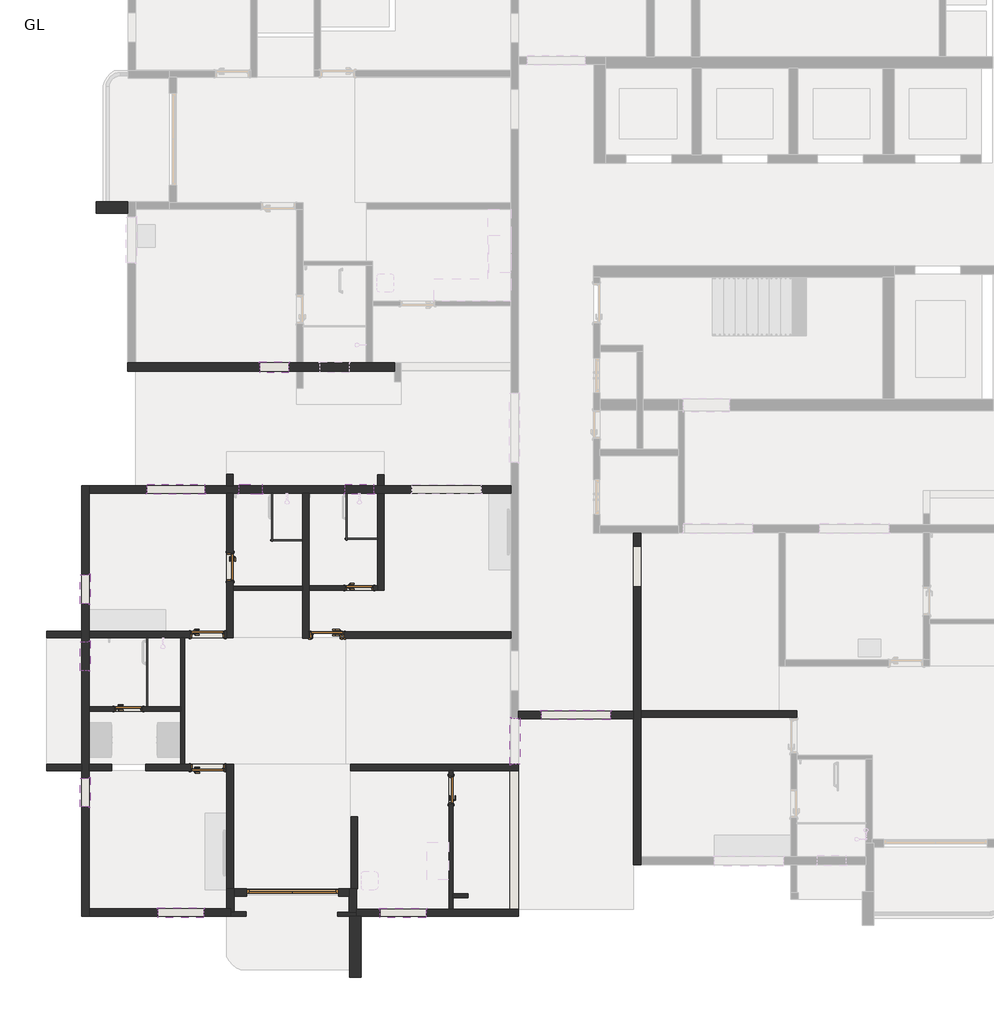
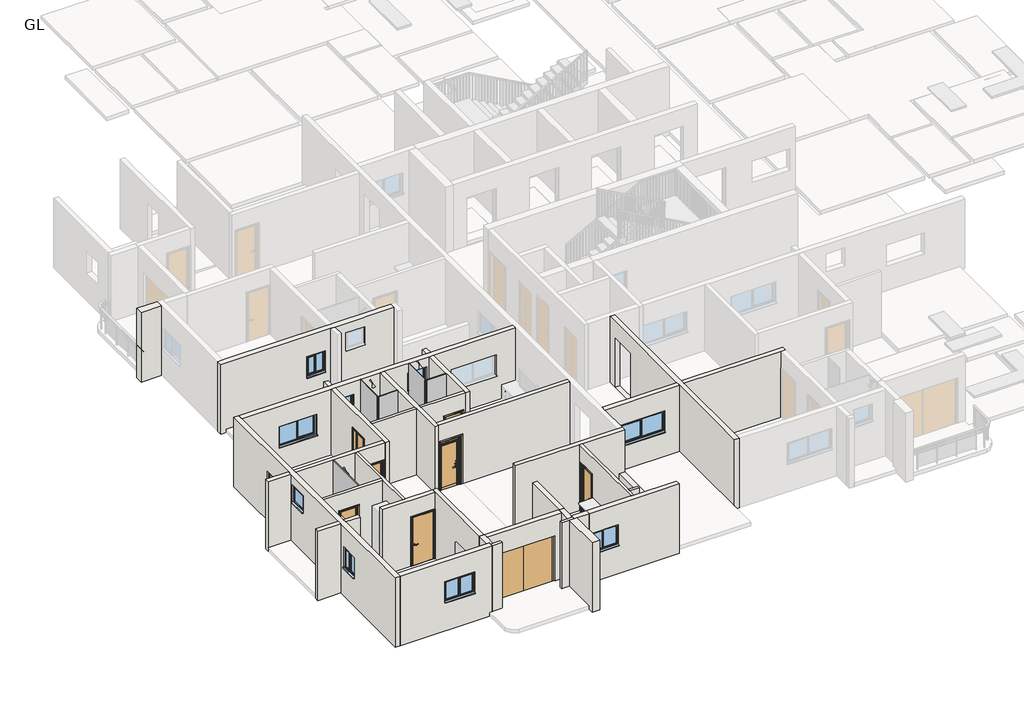
# One storey, part 1 of 14: 36 walls, 11 windows, 9 doors, 5 plates.
"""IFC4 building model written with IfcOpenShell, lengths in millimetres."""

from ifc_helpers import new_model, si_unit, frame, origin, origin_with_axes, place, context, project, spatial, polyline, outline, extrude, faceted_brep, transform, mapped, element, save
from components import doors_concept_extdbl_8_c180431f, doors_intsgl_2_5_door_21b53886, doors_intsgl_2_5_door_ce04bd24, doors_intsgl_2_5_door_1f5f3f16, doors_intsgl_3_door_8261d8fb, doors_intsgl_3_door_f61d7fb9, doors_intsgl_810x2110mm_f0bad3dc, system_panel_glazed_ef83883b, system_panel_glazed_cb88c06f, system_panel_glazed_4b9268f2, system_panel_glazed_6dd91efc, system_panel_glazed_b6b14daa, windows_dbl_plain_2_5_52f1e8c5, windows_dbl_plain_2_5_5b7baf13, windows_dbl_plain_4_4d10fa92, windows_dbl_plain_4_e08ba9e4, windows_dbl_plain_5_c7724a63, windows_dbl_plain_6_decf5736, windows_sgl_plain_2_82341a49, windows_sgl_plain_2_5_9e76a6e6

model = new_model("IFC4")

# Units and contexts
model_context = context("Model", 3, world=origin())
ifc_project = project(units=[si_unit("LENGTHUNIT", "METRE", prefix="MILLI")], contexts=[model_context])

# Site, building, storey
site = spatial("IfcSite", under=ifc_project)
building = spatial("IfcBuilding", under=site)
storey = spatial("IfcBuildingStorey", under=building, Name="GL", Elevation=0.0)

# Doors
placement = place(None, origin())
doors_concept_extdbl_8_shape = doors_concept_extdbl_8_c180431f(model_context)
element("IfcDoor", 1, ObjectType="Doors_Concept_ExtDbl : 8'", at=placement, inside=storey, context=model_context, shape_type="MappedRepresentation", body=[
    mapped(doors_concept_extdbl_8_shape, transform((-11289.2163581, 56773.1334152, 0.0), x_axis=(1.0, 0.0, 0.0), y_axis=(0.0, 1.0, 0.0), z_axis=(0.0, 0.0, 1.0))),
])
doors_intsgl_2_5_door_shape = doors_intsgl_2_5_door_21b53886(model_context)
element("IfcDoor", 2, ObjectType="Doors_IntSgl : 2.5' DOOR", at=placement, inside=storey, context=model_context, shape_type="MappedRepresentation", body=[
    mapped(doors_intsgl_2_5_door_shape, transform((-9514.2506601, 64858.96013, 149.9616), x_axis=(1.0, 0.0, 0.0), y_axis=(0.0, 1.0, 0.0), z_axis=(0.0, 0.0, 1.0))),
])
element("IfcDoor", 3, ObjectType="Doors_IntSgl : 2.5' DOOR", at=placement, inside=storey, context=model_context, shape_type="MappedRepresentation", body=[
    mapped(doors_intsgl_2_5_door_shape, transform((-15646.0698866, 61645.6195727, 149.9616), x_axis=(1.0, 0.0, 0.0), y_axis=(0.0, 1.0, 0.0), z_axis=(0.0, 0.0, 1.0))),
])
doors_intsgl_2_5_door_2_shape = doors_intsgl_2_5_door_ce04bd24(model_context)
element("IfcDoor", 4, ObjectType="Doors_IntSgl : 2.5' DOOR", at=placement, inside=storey, context=model_context, shape_type="MappedRepresentation", body=[
    mapped(doors_intsgl_2_5_door_2_shape, transform((-12951.3420711, 65416.49013, 149.9616), x_axis=(0.0, -1.0, 0.0), y_axis=(1.0, 0.0, 0.0), z_axis=(0.0, 0.0, 1.0))),
])
doors_intsgl_2_5_door_3_shape = doors_intsgl_2_5_door_1f5f3f16(model_context)
element("IfcDoor", 5, ObjectType="Doors_IntSgl : 2.5' DOOR", at=placement, inside=storey, context=model_context, shape_type="MappedRepresentation", body=[
    mapped(doors_intsgl_2_5_door_3_shape, transform((-7083.0672689, 59496.0127724, 149.9616), x_axis=(0.0, 1.0, 0.0), y_axis=(-1.0, 0.0, 0.0), z_axis=(0.0, 0.0, 1.0))),
])
doors_intsgl_3_door_shape = doors_intsgl_3_door_8261d8fb(model_context)
element("IfcDoor", 6, ObjectType="Doors_IntSgl : 3' DOOR", at=placement, inside=storey, context=model_context, shape_type="MappedRepresentation", body=[
    mapped(doors_intsgl_3_door_shape, transform((-13541.6798866, 60093.6754152, 149.9616), x_axis=(1.0, 0.0, 0.0), y_axis=(0.0, 1.0, 0.0), z_axis=(0.0, 0.0, 1.0))),
])
element("IfcDoor", 7, ObjectType="Doors_IntSgl : 3' DOOR", at=placement, inside=storey, context=model_context, shape_type="MappedRepresentation", body=[
    mapped(doors_intsgl_3_door_shape, transform((-10370.9762852, 63608.7807724, 149.9616), x_axis=(-1.0, 0.0, 0.0), y_axis=(0.0, -1.0, 0.0), z_axis=(0.0, 0.0, 1.0))),
])
doors_intsgl_3_door_2_shape = doors_intsgl_3_door_f61d7fb9(model_context)
element("IfcDoor", 8, ObjectType="Doors_IntSgl : 3' DOOR", at=placement, inside=storey, context=model_context, shape_type="MappedRepresentation", body=[
    mapped(doors_intsgl_3_door_2_shape, transform((-13546.2100711, 63618.6686976, 149.9616), x_axis=(1.0, 0.0, 0.0), y_axis=(0.0, 1.0, 0.0), z_axis=(0.0, 0.0, 1.0))),
])
doors_intsgl_810x2110mm_shape = doors_intsgl_810x2110mm_f0bad3dc(model_context)
element("IfcDoor", 9, ObjectType="Doors_IntSgl : 810x2110mm", at=placement, inside=storey, context=model_context, shape_type="MappedRepresentation", body=[
    mapped(doors_intsgl_810x2110mm_shape, transform((-10397.7762852, 63608.7807724, 0.0), x_axis=(-1.0, 0.0, 0.0), y_axis=(0.0, -1.0, 0.0), z_axis=(0.0, 0.0, 1.0))),
])

# Plates
system_panel_glazed_shape = system_panel_glazed_ef83883b(model_context)
element("IfcPlate", 10, ObjectType="System Panel : Glazed", at=placement, inside=storey, context=model_context, shape_type="MappedRepresentation", body=[
    mapped(system_panel_glazed_shape, transform((-11866.147169, 66729.9034152, 0.0), x_axis=(0.0, -1.0, 0.0), y_axis=(1.0, 0.0, 0.0), z_axis=(0.0, 0.0, 1.0))),
])
system_panel_glazed_2_shape = system_panel_glazed_cb88c06f(model_context)
element("IfcPlate", 11, ObjectType="System Panel : Glazed", at=placement, inside=storey, context=model_context, shape_type="MappedRepresentation", body=[
    mapped(system_panel_glazed_2_shape, transform((-11446.7297271, 66092.3334152, 0.0), x_axis=(1.0, 0.0, 0.0), y_axis=(0.0, 1.0, 0.0), z_axis=(0.0, 0.0, 1.0))),
])
system_panel_glazed_3_shape = system_panel_glazed_4b9268f2(model_context)
element("IfcPlate", 12, ObjectType="System Panel : Glazed", at=placement, inside=storey, context=model_context, shape_type="MappedRepresentation", body=[
    mapped(system_panel_glazed_3_shape, transform((-9895.2506601, 66745.1734152, 0.0), x_axis=(0.0, -1.0, 0.0), y_axis=(1.0, 0.0, 0.0), z_axis=(0.0, 0.0, 1.0))),
])
system_panel_glazed_4_shape = system_panel_glazed_6dd91efc(model_context)
element("IfcPlate", 13, ObjectType="System Panel : Glazed", at=placement, inside=storey, context=model_context, shape_type="MappedRepresentation", body=[
    mapped(system_panel_glazed_4_shape, transform((-9463.4506601, 66122.8734152, 0.0), x_axis=(1.0, 0.0, 0.0), y_axis=(0.0, 1.0, 0.0), z_axis=(0.0, 0.0, 1.0))),
])
system_panel_glazed_5_shape = system_panel_glazed_b6b14daa(model_context)
element("IfcPlate", 14, ObjectType="System Panel : Glazed", at=placement, inside=storey, context=model_context, shape_type="MappedRepresentation", body=[
    mapped(system_panel_glazed_5_shape, transform((-15187.4698866, 62623.3346976, 0.0), x_axis=(0.0, -1.0, 0.0), y_axis=(1.0, 0.0, 0.0), z_axis=(0.0, 0.0, 1.0))),
])

# Walls
element("IfcWall", 15, ObjectType="W2", at=placement, inside=storey, context=model_context, shape_type="Brep", body=[
    faceted_brep([(-5294.6931346, 60177.7487724, 3000.0), (-5294.6931346, 60177.7487724, 2110.0), (-5294.6931346, 60177.7487724, 1200.0), (-5294.6931346, 60177.7487724, 0.0), (-5492.8131346, 60177.7487724, 0.0), (-9752.3931346, 60177.7487724, 0.0), (-9752.3931346, 60177.7487724, 3000.0), (-5492.8131346, 60177.7487724, 3000.0), (-5294.6931346, 60004.0127724, 0.0), (-5294.6931346, 60004.0127724, 3000.0), (-7025.9172689, 60004.0127724, 3000.0), (-7140.2172689, 60004.0127724, 3000.0), (-9752.3931346, 60004.0127724, 3000.0), (-9752.3931346, 60004.0127724, 0.0), (-7140.2172689, 60004.0127724, 0.0), (-7025.9172689, 60004.0127724, 0.0), (-5520.9672689, 60004.0127724, 0.0)], [[[0, 1, 2, 3, 4, 5, 6, 7]], [[8, 9, 10, 11, 12, 13, 14, 15, 16]], [[5, 4, 3, 8, 16, 15, 14, 13]], [[6, 5, 13, 12]], [[0, 7, 6, 12, 11, 10, 9]], [[0, 9, 8, 3, 2, 1]]]),
])
element("IfcWall", 16, ObjectType="W2", at=placement, inside=storey, context=model_context, shape_type="Brep", body=[
    faceted_brep([(-9742.8728296, 58794.5197223, 0.0), (-9742.8728296, 56872.1934152, 0.0), (-9742.8728296, 56872.1934152, 3000.0), (-9742.8728296, 58794.5197223, 3000.0), (-9569.1368296, 58794.5197223, 0.0), (-9569.1368296, 58794.5197223, 3000.0), (-9569.1368296, 56872.1934152, 3000.0), (-9569.1368296, 56872.1934152, 0.0), (-9585.6556011, 56872.1934152, 0.0), (-9585.6556011, 56872.1934152, 3000.0)], [[[0, 1, 2, 3]], [[4, 5, 6, 7]], [[1, 0, 4, 7, 8]], [[3, 2, 9, 6, 5]], [[0, 3, 5, 4]], [[2, 1, 8, 7, 6, 9]]]),
])
element("IfcWall", 17, ObjectType="W2", at=placement, inside=storey, context=model_context, shape_type="Brep", body=[
    faceted_brep([(-12859.9438866, 56872.1934152, 0.0), (-12859.9438866, 60180.5434152, 0.0), (-12859.9438866, 60180.5434152, 3000.0), (-12859.9438866, 56872.1934152, 3000.0), (-13033.6798866, 56872.1934152, 0.0), (-13033.6798866, 56872.1934152, 3000.0), (-13033.6798866, 60006.8074152, 3000.0), (-13033.6798866, 60180.5434152, 3000.0), (-13033.6798866, 60180.5434152, 0.0), (-13033.6798866, 60006.8074152, 0.0)], [[[0, 1, 2, 3]], [[4, 5, 6, 7, 8, 9]], [[1, 0, 4, 9, 8]], [[3, 2, 7, 6, 5]], [[0, 3, 5, 4]], [[2, 1, 8, 7]]]),
])
element("IfcWall", 18, ObjectType="W2", at=placement, inside=storey, context=model_context, shape_type="Brep", body=[
    faceted_brep([(-13033.6798866, 60180.5434152, 0.0), (-14151.3407376, 60180.5434152, 0.0), (-14265.6407376, 60180.5434152, 0.0), (-15194.7118866, 60180.5434152, 0.0), (-15194.7118866, 60180.5434152, 3000.0), (-14265.6407376, 60180.5434152, 3000.0), (-14151.3407376, 60180.5434152, 3000.0), (-13033.6798866, 60180.5434152, 3000.0), (-13084.4798866, 60180.5434152, 149.9616), (-13084.4798866, 60180.5434152, 2259.9616), (-13998.8798866, 60180.5434152, 2259.9616), (-13998.8798866, 60180.5434152, 149.9616), (-15194.7118866, 60006.8074152, 0.0), (-13033.6798866, 60006.8074152, 0.0), (-13033.6798866, 60006.8074152, 3000.0), (-15194.7118866, 60006.8074152, 3000.0), (-13084.4798866, 60006.8074152, 2259.9616), (-13084.4798866, 60006.8074152, 149.9616), (-13998.8798866, 60006.8074152, 149.9616), (-13998.8798866, 60006.8074152, 2259.9616)], [[[0, 1, 2, 3, 4, 5, 6, 7], [8, 9, 10, 11]], [[12, 13, 14, 15], [16, 17, 18, 19]], [[3, 2, 1, 0, 13, 12]], [[4, 3, 12, 15]], [[7, 6, 5, 4, 15, 14]], [[0, 7, 14, 13]], [[8, 17, 16, 9]], [[9, 16, 19, 10]], [[10, 19, 18, 11]], [[17, 8, 11, 18]]]),
])
element("IfcWall", 19, ObjectType="W2", at=placement, inside=storey, context=model_context, shape_type="SweptSolid", body=[
    extrude(outline(polyline([(-17819.0398866, 63705.5366976), (-16889.3998866, 63705.5366976), (-16889.3998866, 63531.8006976), (-17819.0398866, 63531.8006976), (-17819.0398866, 63705.5366976)])), origin_with_axes(), (0.0, 0.0, 1.0), 3000.0),
])
element("IfcWall", 20, ObjectType="W2", at=placement, inside=storey, context=model_context, shape_type="Brep", body=[
    faceted_brep([(-13038.2100711, 67367.4734152, 0.0), (-13038.2100711, 63705.5366976, 0.0), (-13038.2100711, 63531.8006976, 0.0), (-13038.2100711, 63531.8006976, 3000.0), (-13038.2100711, 63705.5366976, 3000.0), (-13038.2100711, 67367.4734152, 3000.0), (-13038.2100711, 65035.49013, 2259.9616), (-13038.2100711, 65035.49013, 149.9616), (-13038.2100711, 65797.49013, 149.9616), (-13038.2100711, 65797.49013, 2259.9616), (-12864.4740711, 63531.8006976, 0.0), (-12864.4740711, 64794.19013, 0.0), (-12864.4740711, 64908.49013, 0.0), (-12864.4740711, 67367.4734152, 0.0), (-12864.4740711, 67367.4734152, 3000.0), (-12864.4740711, 64908.49013, 3000.0), (-12864.4740711, 64794.19013, 3000.0), (-12864.4740711, 63531.8006976, 3000.0), (-12864.4740711, 65035.49013, 149.9616), (-12864.4740711, 65035.49013, 2259.9616), (-12864.4740711, 65797.49013, 2259.9616), (-12864.4740711, 65797.49013, 149.9616)], [[[0, 1, 2, 3, 4, 5], [6, 7, 8, 9]], [[10, 11, 12, 13, 14, 15, 16, 17], [18, 19, 20, 21]], [[2, 1, 0, 13, 12, 11, 10]], [[5, 4, 3, 17, 16, 15, 14]], [[0, 5, 14, 13]], [[3, 2, 10, 17]], [[18, 7, 6, 19]], [[19, 6, 9, 20]], [[20, 9, 8, 21]], [[7, 18, 21, 8]]]),
])
element("IfcWall", 21, ObjectType="W2", at=placement, inside=storey, context=model_context, shape_type="Brep", body=[
    faceted_brep([(-11027.3122852, 67367.4734152, 0.0), (-11027.3122852, 64908.49013, 0.0), (-11027.3122852, 64794.19013, 0.0), (-11027.3122852, 63521.9127724, 0.0), (-11027.3122852, 63521.9127724, 3000.0), (-11027.3122852, 64794.19013, 3000.0), (-11027.3122852, 64908.49013, 3000.0), (-11027.3122852, 67367.4734152, 3000.0), (-10853.5762852, 67367.4734152, 0.0), (-10853.5762852, 67367.4734152, 3000.0), (-10853.5762852, 64916.11013, 3000.0), (-10853.5762852, 64801.81013, 3000.0), (-10853.5762852, 63695.6487724, 3000.0), (-10853.5762852, 63521.9127724, 3000.0), (-10853.5762852, 63521.9127724, 0.0), (-10853.5762852, 63695.6487724, 0.0), (-10853.5762852, 64801.81013, 0.0), (-10853.5762852, 64916.11013, 0.0)], [[[0, 1, 2, 3, 4, 5, 6, 7]], [[8, 9, 10, 11, 12, 13, 14, 15, 16, 17]], [[3, 2, 1, 0, 8, 17, 16, 15, 14]], [[7, 6, 5, 4, 13, 12, 11, 10, 9]], [[0, 7, 9, 8]], [[4, 3, 14, 13]]]),
])
element("IfcWall", 22, ObjectType="W2", at=placement, inside=storey, context=model_context, shape_type="Brep", body=[
    faceted_brep([(-9031.6506601, 67367.4734152, 0.0), (-9031.6506601, 64916.11013, 0.0), (-9031.6506601, 64801.81013, 0.0), (-9031.6506601, 64801.81013, 3000.0), (-9031.6506601, 64916.11013, 3000.0), (-9031.6506601, 67367.4734152, 3000.0), (-8857.9146601, 67367.4734152, 0.0), (-8857.9146601, 67367.4734152, 3000.0), (-8857.9146601, 64801.81013, 3000.0), (-8857.9146601, 64801.81013, 0.0)], [[[0, 1, 2, 3, 4, 5]], [[6, 7, 8, 9]], [[2, 1, 0, 6, 9]], [[5, 4, 3, 8, 7]], [[0, 5, 7, 6]], [[3, 2, 9, 8]]]),
])
element("IfcWall", 23, ObjectType="W2", at=placement, inside=storey, context=model_context, shape_type="SweptSolid", body=[
    extrude(outline(polyline([(3000.0, -5492.8131346), (3000.0, -10853.5762852), (0.0, -10853.5762852), (0.0, -10802.7762852), (149.9616, -10802.7762852), (149.9616, -10828.1762852), (2259.9616, -10828.1762852), (2259.9616, -9913.7762852), (149.9616, -9913.7762852), (149.9616, -9992.7762852), (0.0, -9992.7762852), (0.0, -5492.8131346), (3000.0, -5492.8131346)])), frame((0.0, 63521.9127724, 0.0), z_axis=(0.0, 1.0, 0.0), x_axis=(0.0, 0.0, 1.0)), (0.0, 0.0, 1.0), 173.736),
])
element("IfcWall", 24, ObjectType="W2", at=placement, inside=storey, context=model_context, shape_type="Brep", body=[
    faceted_brep([(-16691.2798866, 63531.8006976, 0.0), (-14265.6407376, 63531.8006976, 0.0), (-14151.3407376, 63531.8006976, 0.0), (-13038.2100711, 63531.8006976, 0.0), (-13038.2100711, 63531.8006976, 3000.0), (-14151.3407376, 63531.8006976, 3000.0), (-14265.6407376, 63531.8006976, 3000.0), (-16691.2798866, 63531.8006976, 3000.0), (-13089.0100711, 63531.8006976, 2259.9616), (-13089.0100711, 63531.8006976, 149.9616), (-14003.4100711, 63531.8006976, 149.9616), (-14003.4100711, 63531.8006976, 2259.9616), (-13038.2100711, 63705.5366976, 0.0), (-16691.2798866, 63705.5366976, 0.0), (-16691.2798866, 63705.5366976, 3000.0), (-13038.2100711, 63705.5366976, 3000.0), (-13089.0100711, 63705.5366976, 149.9616), (-13089.0100711, 63705.5366976, 2259.9616), (-14003.4100711, 63705.5366976, 2259.9616), (-14003.4100711, 63705.5366976, 149.9616)], [[[0, 1, 2, 3, 4, 5, 6, 7], [8, 9, 10, 11]], [[12, 13, 14, 15], [16, 17, 18, 19]], [[3, 2, 1, 0, 13, 12]], [[7, 6, 5, 4, 15, 14]], [[0, 7, 14, 13]], [[4, 3, 12, 15]], [[16, 9, 8, 17]], [[17, 8, 11, 18]], [[18, 11, 10, 19]], [[9, 16, 19, 10]]]),
])
element("IfcWall", 25, ObjectType="W2", at=placement, inside=storey, context=model_context, shape_type="SweptSolid", body=[
    extrude(outline(polyline([(-17820.0558866, 60006.8074152), (-17820.0558866, 60180.5434152), (-16889.3998866, 60180.5434152), (-16889.3998866, 60006.8074152), (-17820.0558866, 60006.8074152)])), origin_with_axes(), (0.0, 0.0, 1.0), 3000.0),
    extrude(outline(polyline([(-16092.8558866, 60180.5434152), (-16092.8558866, 60006.8074152), (-16691.2798866, 60006.8074152), (-16691.2798866, 60180.5434152), (-16092.8558866, 60180.5434152)])), origin_with_axes(), (0.0, 0.0, 1.0), 3000.0),
])
element("IfcWall", 26, ObjectType="W2", at=placement, inside=storey, context=model_context, shape_type="SweptSolid", body=[
    extrude(outline(polyline([(-12864.4740711, 67870.3934152), (-12864.4740711, 67565.5934152), (-13038.2100711, 67565.5934152), (-13038.2100711, 67870.3934152), (-12864.4740711, 67870.3934152)])), origin_with_axes(), (0.0, 0.0, 1.0), 3000.0),
])
element("IfcWall", 27, ObjectType="W2", at=placement, inside=storey, context=model_context, shape_type="SweptSolid", body=[
    extrude(outline(polyline([(-8857.9146601, 67864.0434152), (-8857.9146601, 67565.5934152), (-9031.6506601, 67565.5934152), (-9031.6506601, 67864.0434152), (-8857.9146601, 67864.0434152)])), origin_with_axes(), (0.0, 0.0, 1.0), 3000.0),
])
element("IfcWall", 28, ObjectType="W2", at=placement, inside=storey, context=model_context, shape_type="Brep", body=[
    faceted_brep([(-2044.3665436, 61430.4767724, 0.0), (1930.5893567, 61430.4767724, 0.0), (2098.2293567, 61430.4767724, 0.0), (2098.2293567, 61430.4767724, 3000.0), (1930.5893567, 61430.4767724, 3000.0), (-2044.3665436, 61430.4767724, 3000.0), (-2044.3665436, 61604.2127724, 0.0), (-2044.3665436, 61604.2127724, 3000.0), (2098.2293567, 61604.2127724, 3000.0), (2098.2293567, 61604.2127724, 0.0)], [[[0, 1, 2, 3, 4, 5]], [[6, 7, 8, 9]], [[2, 1, 0, 6, 9]], [[5, 4, 3, 8, 7]], [[0, 5, 7, 6]], [[3, 2, 9, 8]]]),
])
element("IfcWall", 29, ObjectType="W3", at=placement, inside=storey, context=model_context, shape_type="SweptSolid", body=[
    extrude(outline(polyline([(0.0, -10853.5762852), (0.0, -9031.6506601), (3000.0, -9031.6506601), (3000.0, -10853.5762852), (0.0, -10853.5762852)]), holes=[polyline([(2259.9616, -9133.2506601), (149.9616, -9133.2506601), (149.9616, -9895.2506601), (2259.9616, -9895.2506601), (2259.9616, -9133.2506601)])]), frame((0.0, 64801.81013, 0.0), z_axis=(0.0, 1.0, 0.0), x_axis=(0.0, 0.0, 1.0)), (0.0, 0.0, 1.0), 114.3),
])
element("IfcWall", 30, ObjectType="W3", at=placement, inside=storey, context=model_context, shape_type="SweptSolid", body=[
    extrude(outline(polyline([(-12864.4740711, 64908.49013), (-11027.3122852, 64908.49013), (-11027.3122852, 64794.19013), (-12864.4740711, 64794.19013), (-12864.4740711, 64908.49013)])), origin_with_axes(), (0.0, 0.0, 1.0), 3000.0),
])
element("IfcWall", 31, ObjectType="W3", at=placement, inside=storey, context=model_context, shape_type="Brep", body=[
    faceted_brep([(-14265.6407376, 63531.8006976, 0.0), (-14265.6407376, 61702.7695727, 0.0), (-14265.6407376, 61588.4695727, 0.0), (-14265.6407376, 60180.5434152, 0.0), (-14265.6407376, 60180.5434152, 3000.0), (-14265.6407376, 61588.4695727, 3000.0), (-14265.6407376, 61702.7695727, 3000.0), (-14265.6407376, 63531.8006976, 3000.0), (-14151.3407376, 63531.8006976, 0.0), (-14151.3407376, 63531.8006976, 3000.0), (-14151.3407376, 60180.5434152, 3000.0), (-14151.3407376, 60180.5434152, 0.0)], [[[0, 1, 2, 3, 4, 5, 6, 7]], [[8, 9, 10, 11]], [[3, 2, 1, 0, 8, 11]], [[7, 6, 5, 4, 10, 9]], [[4, 3, 11, 10]], [[0, 7, 9, 8]]]),
])
element("IfcWall", 32, ObjectType="W3", at=placement, inside=storey, context=model_context, shape_type="SweptSolid", body=[
    extrude(outline(polyline([(0.0, -16691.2798866), (0.0, -14265.6407376), (3000.0, -14265.6407376), (3000.0, -16691.2798866), (0.0, -16691.2798866)]), holes=[polyline([(2259.9616, -15265.0698866), (149.9616, -15265.0698866), (149.9616, -16027.0698866), (2259.9616, -16027.0698866), (2259.9616, -15265.0698866)])]), frame((0.0, 61588.4695727, 0.0), z_axis=(0.0, 1.0, 0.0), x_axis=(0.0, 0.0, 1.0)), (0.0, 0.0, 1.0), 114.3),
])
element("IfcWall", 33, ObjectType="W3", at=placement, inside=storey, context=model_context, shape_type="Brep", body=[
    faceted_brep([(-12524.4098866, 56265.3874152, 0.0), (-12835.5598866, 56265.3874152, 0.0), (-12934.6198866, 56265.3874152, 0.0), (-12934.6198866, 56265.3874152, 3000.0), (-12835.5598866, 56265.3874152, 3000.0), (-12524.4098866, 56265.3874152, 3000.0), (-12524.4098866, 56151.0874152, 0.0), (-12524.4098866, 56151.0874152, 3000.0), (-12934.6198866, 56151.0874152, 3000.0), (-12934.6198866, 56151.0874152, 0.0)], [[[0, 1, 2, 3, 4, 5]], [[6, 7, 8, 9]], [[2, 1, 0, 6, 9]], [[3, 2, 9, 8]], [[5, 4, 3, 8, 7]], [[0, 5, 7, 6]]]),
])
element("IfcWall", 34, ObjectType="W3", at=placement, inside=storey, context=model_context, shape_type="Brep", body=[
    faceted_brep([(-9585.6556011, 56257.2296151, 0.0), (-9783.7756011, 56257.2296151, 0.0), (-10094.9256011, 56257.2296151, 0.0), (-10094.9256011, 56257.2296151, 3000.0), (-9783.7756011, 56257.2296151, 3000.0), (-9585.6556011, 56257.2296151, 3000.0), (-9585.6556011, 56142.9296151, 0.0), (-9585.6556011, 56142.9296151, 3000.0), (-9782.0683526, 56142.9296151, 3000.0), (-10094.9256011, 56142.9296151, 3000.0), (-10094.9256011, 56142.9296151, 0.0), (-9782.0683526, 56142.9296151, 0.0)], [[[0, 1, 2, 3, 4, 5]], [[6, 7, 8, 9, 10, 11]], [[2, 1, 0, 6, 11, 10]], [[3, 2, 10, 9]], [[5, 4, 3, 9, 8, 7]], [[0, 5, 7, 6]]]),
])
element("IfcWall", 35, ObjectType="W3", at=placement, inside=storey, context=model_context, shape_type="Brep", body=[
    faceted_brep([(-7025.9172689, 56341.0496151, 0.0), (-7025.9172689, 56636.5035386, 0.0), (-7025.9172689, 56750.8035386, 0.0), (-7025.9172689, 60004.0127724, 0.0), (-7025.9172689, 60004.0127724, 3000.0), (-7025.9172689, 56750.8035386, 3000.0), (-7025.9172689, 56636.5035386, 3000.0), (-7025.9172689, 56341.0496151, 3000.0), (-7025.9172689, 59877.0127724, 2259.9616), (-7025.9172689, 59877.0127724, 149.9616), (-7025.9172689, 59115.0127724, 149.9616), (-7025.9172689, 59115.0127724, 2259.9616), (-7140.2172689, 60004.0127724, 0.0), (-7140.2172689, 56341.0496151, 0.0), (-7140.2172689, 56341.0496151, 3000.0), (-7140.2172689, 60004.0127724, 3000.0), (-7140.2172689, 59877.0127724, 149.9616), (-7140.2172689, 59877.0127724, 2259.9616), (-7140.2172689, 59115.0127724, 2259.9616), (-7140.2172689, 59115.0127724, 149.9616)], [[[0, 1, 2, 3, 4, 5, 6, 7], [8, 9, 10, 11]], [[12, 13, 14, 15], [16, 17, 18, 19]], [[3, 2, 1, 0, 13, 12]], [[7, 6, 5, 4, 15, 14]], [[4, 3, 12, 15]], [[0, 7, 14, 13]], [[16, 9, 8, 17]], [[17, 8, 11, 18]], [[18, 11, 10, 19]], [[9, 16, 19, 10]]]),
])
element("IfcWall", 36, ObjectType="W3", at=placement, inside=storey, context=model_context, shape_type="SweptSolid", body=[
    extrude(outline(polyline([(-6632.2172689, 56636.5035386), (-7025.9172689, 56636.5035386), (-7025.9172689, 56750.8035386), (-6632.2172689, 56750.8035386), (-6632.2172689, 56636.5035386)])), origin_with_axes(), (0.0, 0.0, 1.0), 3000.0),
])
element("IfcWall", 37, ObjectType="W4", at=placement, inside=storey, context=model_context, shape_type="Brep", body=[
    faceted_brep([(-9477.2683526, 54525.5707921, 0.0), (-9477.2683526, 56142.9296151, 0.0), (-9477.2683526, 56142.9296151, 3000.0), (-9477.2683526, 54525.5707921, 3000.0), (-9782.0683526, 54525.5707921, 0.0), (-9782.0683526, 54525.5707921, 3000.0), (-9782.0683526, 56142.9296151, 3000.0), (-9782.0683526, 56142.9296151, 0.0), (-9585.6556011, 56142.9296151, 0.0), (-9585.6556011, 56142.9296151, 3000.0)], [[[0, 1, 2, 3]], [[4, 5, 6, 7]], [[1, 0, 4, 7, 8]], [[3, 2, 9, 6, 5]], [[0, 3, 5, 4]], [[2, 1, 8, 7, 6, 9]]]),
])
element("IfcWall", 38, ObjectType="W4", at=placement, inside=storey, context=model_context, shape_type="SweptSolid", body=[
    extrude(outline(polyline([(-15665.5131346, 74800.7827724), (-16503.7131346, 74800.7827724), (-16503.7131346, 75105.5827724), (-15665.5131346, 75105.5827724), (-15665.5131346, 74800.7827724)])), origin_with_axes(), (0.0, 0.0, 1.0), 3000.0),
])
element("IfcWall", 39, ObjectType="W5", at=placement, inside=storey, context=model_context, shape_type="Brep", body=[
    faceted_brep([(-5292.3672689, 56341.0496151, 0.0), (-5292.3672689, 60004.0127724, 0.0), (-5292.3672689, 60004.0127724, 1171.2), (-5292.3672689, 56341.0496151, 1171.2), (-5520.9672689, 56341.0496151, 0.0), (-5520.9672689, 56341.0496151, 1171.2), (-5520.9672689, 60004.0127724, 1171.2), (-5520.9672689, 60004.0127724, 0.0), (-5294.6931346, 60004.0127724, 0.0)], [[[0, 1, 2, 3]], [[4, 5, 6, 7]], [[1, 0, 4, 7, 8]], [[3, 2, 6, 5]], [[0, 3, 5, 4]], [[2, 1, 8, 7, 6]]]),
])
element("IfcWall", 40, ObjectType="W5", at=placement, inside=storey, context=model_context, shape_type="Brep", body=[
    faceted_brep([(-8587.5491346, 70838.3827724, 0.0), (-9163.1131346, 70838.3827724, 0.0), (-9336.8491346, 70838.3827724, 0.0), (-11010.9631346, 70838.3827724, 0.0), (-11178.6031346, 70838.3827724, 0.0), (-15452.1531346, 70838.3827724, 0.0), (-15665.5131346, 70838.3827724, 0.0), (-15665.5131346, 70838.3827724, 3000.0), (-15452.1531346, 70838.3827724, 3000.0), (-11178.6031346, 70838.3827724, 3000.0), (-11010.9631346, 70838.3827724, 3000.0), (-9336.8491346, 70838.3827724, 3000.0), (-9163.1131346, 70838.3827724, 3000.0), (-8587.5491346, 70838.3827724, 3000.0), (-9794.0491346, 70838.3827724, 2590.8), (-10556.0491346, 70838.3827724, 2590.8), (-10556.0491346, 70838.3827724, 1828.8), (-9794.0491346, 70838.3827724, 1828.8), (-11394.2491346, 70838.3827724, 2110.0), (-12156.2491346, 70838.3827724, 2110.0), (-12156.2491346, 70838.3827724, 1200.0), (-11394.2491346, 70838.3827724, 1200.0), (-8587.5491346, 70609.7827724, 0.0), (-8587.5491346, 70609.7827724, 3000.0), (-11010.9631346, 70609.7827724, 3000.0), (-11178.6031346, 70609.7827724, 3000.0), (-15665.5131346, 70609.7827724, 3000.0), (-15665.5131346, 70609.7827724, 0.0), (-11178.6031346, 70609.7827724, 0.0), (-11010.9631346, 70609.7827724, 0.0), (-9794.0491346, 70609.7827724, 2590.8), (-9794.0491346, 70609.7827724, 1828.8), (-10556.0491346, 70609.7827724, 1828.8), (-10556.0491346, 70609.7827724, 2590.8), (-11394.2491346, 70609.7827724, 2110.0), (-11394.2491346, 70609.7827724, 1200.0), (-12156.2491346, 70609.7827724, 1200.0), (-12156.2491346, 70609.7827724, 2110.0)], [[[0, 1, 2, 3, 4, 5, 6, 7, 8, 9, 10, 11, 12, 13], [14, 15, 16, 17], [18, 19, 20, 21]], [[22, 23, 24, 25, 26, 27, 28, 29], [30, 31, 32, 33], [34, 35, 36, 37]], [[6, 5, 4, 3, 2, 1, 0, 22, 29, 28, 27]], [[13, 12, 11, 10, 9, 8, 7, 26, 25, 24, 23]], [[7, 6, 27, 26]], [[31, 30, 14, 17]], [[32, 31, 17, 16]], [[33, 32, 16, 15]], [[30, 33, 15, 14]], [[35, 34, 18, 21]], [[36, 35, 21, 20]], [[37, 36, 20, 19]], [[34, 37, 19, 18]], [[0, 13, 23, 22]]]),
])
element("IfcWall", 41, ObjectType="WALL 1", at=placement, inside=storey, context=model_context, shape_type="Brep", body=[
    faceted_brep([(-16691.2798866, 56151.0874152, 0.0), (-16691.2798866, 56349.2074152, 0.0), (-16691.2798866, 60006.8074152, 0.0), (-16691.2798866, 60180.5434152, 0.0), (-16691.2798866, 61588.4695727, 0.0), (-16691.2798866, 61702.7695727, 0.0), (-16691.2798866, 63531.8006976, 0.0), (-16691.2798866, 63705.5366976, 0.0), (-16691.2798866, 67367.4734152, 0.0), (-16691.2798866, 67565.5934152, 0.0), (-16691.2798866, 67565.5934152, 3000.0), (-16691.2798866, 67367.4734152, 3000.0), (-16691.2798866, 63705.5366976, 3000.0), (-16691.2798866, 63531.8006976, 3000.0), (-16691.2798866, 61702.7695727, 3000.0), (-16691.2798866, 61588.4695727, 3000.0), (-16691.2798866, 60180.5434152, 3000.0), (-16691.2798866, 60006.8074152, 3000.0), (-16691.2798866, 56349.2074152, 3000.0), (-16691.2798866, 56151.0874152, 3000.0), (-16691.2798866, 59048.4695727, 2110.0), (-16691.2798866, 59810.4695727, 2110.0), (-16691.2798866, 59810.4695727, 1200.0), (-16691.2798866, 59048.4695727, 1200.0), (-16691.2798866, 62668.2006976, 2590.8), (-16691.2798866, 63430.2006976, 2590.8), (-16691.2798866, 63430.2006976, 1828.8), (-16691.2798866, 62668.2006976, 1828.8), (-16691.2798866, 64442.1366976, 2110.0), (-16691.2798866, 65204.1366976, 2110.0), (-16691.2798866, 65204.1366976, 1200.0), (-16691.2798866, 64442.1366976, 1200.0), (-16889.3998866, 56151.0874152, 0.0), (-16889.3998866, 56151.0874152, 3000.0), (-16889.3998866, 60006.8074152, 3000.0), (-16889.3998866, 60180.5434152, 3000.0), (-16889.3998866, 63531.8006976, 3000.0), (-16889.3998866, 63705.5366976, 3000.0), (-16889.3998866, 67565.5934152, 3000.0), (-16889.3998866, 67565.5934152, 0.0), (-16889.3998866, 63705.5366976, 0.0), (-16889.3998866, 63531.8006976, 0.0), (-16889.3998866, 60180.5434152, 0.0), (-16889.3998866, 60006.8074152, 0.0), (-16889.3998866, 59048.4695727, 2110.0), (-16889.3998866, 59048.4695727, 1200.0), (-16889.3998866, 59810.4695727, 1200.0), (-16889.3998866, 59810.4695727, 2110.0), (-16889.3998866, 62668.2006976, 2590.8), (-16889.3998866, 62668.2006976, 1828.8), (-16889.3998866, 63430.2006976, 1828.8), (-16889.3998866, 63430.2006976, 2590.8), (-16889.3998866, 64442.1366976, 2110.0), (-16889.3998866, 64442.1366976, 1200.0), (-16889.3998866, 65204.1366976, 1200.0), (-16889.3998866, 65204.1366976, 2110.0)], [[[0, 1, 2, 3, 4, 5, 6, 7, 8, 9, 10, 11, 12, 13, 14, 15, 16, 17, 18, 19], [20, 21, 22, 23], [24, 25, 26, 27], [28, 29, 30, 31]], [[32, 33, 34, 35, 36, 37, 38, 39, 40, 41, 42, 43], [44, 45, 46, 47], [48, 49, 50, 51], [52, 53, 54, 55]], [[9, 8, 7, 6, 5, 4, 3, 2, 1, 0, 32, 43, 42, 41, 40, 39]], [[19, 18, 17, 16, 15, 14, 13, 12, 11, 10, 38, 37, 36, 35, 34, 33]], [[0, 19, 33, 32]], [[10, 9, 39, 38]], [[45, 44, 20, 23]], [[46, 45, 23, 22]], [[47, 46, 22, 21]], [[44, 47, 21, 20]], [[49, 48, 24, 27]], [[50, 49, 27, 26]], [[51, 50, 26, 25]], [[48, 51, 25, 24]], [[53, 52, 28, 31]], [[54, 53, 31, 30]], [[55, 54, 30, 29]], [[52, 55, 29, 28]]]),
])
element("IfcWall", 42, ObjectType="WALL 1", at=placement, inside=storey, context=model_context, shape_type="Brep", body=[
    faceted_brep([(-16691.2798866, 56151.0874152, 0.0), (-12934.6198866, 56151.0874152, 0.0), (-12934.6198866, 56151.0874152, 3000.0), (-16691.2798866, 56151.0874152, 3000.0), (-14862.4798866, 56151.0874152, 2110.0), (-13643.2798866, 56151.0874152, 2110.0), (-13643.2798866, 56151.0874152, 1200.0), (-14862.4798866, 56151.0874152, 1200.0), (-16691.2798866, 56349.2074152, 0.0), (-16691.2798866, 56349.2074152, 3000.0), (-13033.6798866, 56349.2074152, 3000.0), (-12934.6198866, 56349.2074152, 3000.0), (-12934.6198866, 56349.2074152, 0.0), (-13033.6798866, 56349.2074152, 0.0), (-14862.4798866, 56349.2074152, 2110.0), (-14862.4798866, 56349.2074152, 1200.0), (-13643.2798866, 56349.2074152, 1200.0), (-13643.2798866, 56349.2074152, 2110.0), (-12934.6198866, 56265.3874152, 0.0), (-12934.6198866, 56265.3874152, 3000.0)], [[[0, 1, 2, 3], [4, 5, 6, 7]], [[8, 9, 10, 11, 12, 13], [14, 15, 16, 17]], [[1, 0, 8, 13, 12, 18]], [[2, 1, 18, 12, 11, 19]], [[3, 2, 19, 11, 10, 9]], [[0, 3, 9, 8]], [[15, 14, 4, 7]], [[16, 15, 7, 6]], [[17, 16, 6, 5]], [[14, 17, 5, 4]]]),
])
element("IfcWall", 43, ObjectType="WALL 1", at=placement, inside=storey, context=model_context, shape_type="Brep", body=[
    faceted_brep([(-12835.5598866, 56265.3874152, 0.0), (-12835.5598866, 56674.0734152, 0.0), (-12835.5598866, 56872.1934152, 0.0), (-12835.5598866, 56872.1934152, 3000.0), (-12835.5598866, 56674.0734152, 3000.0), (-12835.5598866, 56265.3874152, 3000.0), (-13033.6798866, 56349.2074152, 0.0), (-13033.6798866, 56349.2074152, 3000.0), (-13033.6798866, 56872.1934152, 3000.0), (-13033.6798866, 56872.1934152, 0.0), (-12934.6198866, 56265.3874152, 0.0), (-12934.6198866, 56349.2074152, 0.0), (-12859.9438866, 56872.1934152, 0.0), (-12859.9438866, 56872.1934152, 3000.0), (-12934.6198866, 56349.2074152, 3000.0), (-12934.6198866, 56265.3874152, 3000.0)], [[[0, 1, 2, 3, 4, 5]], [[6, 7, 8, 9]], [[2, 1, 0, 10, 11, 6, 9, 12]], [[5, 4, 3, 13, 8, 7, 14, 15]], [[3, 2, 12, 9, 8, 13]], [[0, 5, 15, 10]], [[15, 14, 11, 10]], [[14, 7, 6, 11]]]),
])
element("IfcWall", 44, ObjectType="WALL 1", at=placement, inside=storey, context=model_context, shape_type="SweptSolid", body=[
    extrude(outline(polyline([(2110.0, -10070.0163581), (0.0, -10070.0163581), (0.0, -9783.7756011), (3000.0, -9783.7756011), (3000.0, -12835.5598866), (0.0, -12835.5598866), (0.0, -12508.4163581), (2110.0, -12508.4163581), (2110.0, -10070.0163581)])), frame((0.0, 56674.0734152, 0.0), z_axis=(0.0, 1.0, 0.0), x_axis=(0.0, 0.0, 1.0)), (0.0, 0.0, 1.0), 198.12),
])
element("IfcWall", 45, ObjectType="WALL 1", at=placement, inside=storey, context=model_context, shape_type="Brep", body=[
    faceted_brep([(-16691.2798866, 67367.4734152, 0.0), (-13038.2100711, 67367.4734152, 0.0), (-12864.4740711, 67367.4734152, 0.0), (-11027.3122852, 67367.4734152, 0.0), (-10853.5762852, 67367.4734152, 0.0), (-9031.6506601, 67367.4734152, 0.0), (-8857.9146601, 67367.4734152, 0.0), (-5492.8131346, 67367.4734152, 0.0), (-5492.8131346, 67367.4734152, 3000.0), (-8857.9146601, 67367.4734152, 3000.0), (-9031.6506601, 67367.4734152, 3000.0), (-10853.5762852, 67367.4734152, 3000.0), (-11027.3122852, 67367.4734152, 3000.0), (-12864.4740711, 67367.4734152, 3000.0), (-13038.2100711, 67367.4734152, 3000.0), (-16691.2798866, 67367.4734152, 3000.0), (-15146.4100711, 67367.4734152, 2110.0), (-13622.4100711, 67367.4734152, 2110.0), (-13622.4100711, 67367.4734152, 1200.0), (-15146.4100711, 67367.4734152, 1200.0), (-12712.0740711, 67367.4734152, 2438.4), (-12102.4740711, 67367.4734152, 2438.4), (-12102.4740711, 67367.4734152, 1828.8), (-12712.0740711, 67367.4734152, 1828.8), (-9895.2506601, 67367.4734152, 2590.8), (-9133.2506601, 67367.4734152, 2590.8), (-9133.2506601, 67367.4734152, 1828.8), (-9895.2506601, 67367.4734152, 1828.8), (-8121.3146601, 67367.4734152, 2110.0), (-6292.5146601, 67367.4734152, 2110.0), (-6292.5146601, 67367.4734152, 1200.0), (-8121.3146601, 67367.4734152, 1200.0), (-16691.2798866, 67565.5934152, 0.0), (-16691.2798866, 67565.5934152, 3000.0), (-13038.2100711, 67565.5934152, 3000.0), (-12864.4740711, 67565.5934152, 3000.0), (-9031.6506601, 67565.5934152, 3000.0), (-8857.9146601, 67565.5934152, 3000.0), (-5492.8131346, 67565.5934152, 3000.0), (-5492.8131346, 67565.5934152, 0.0), (-8857.9146601, 67565.5934152, 0.0), (-9031.6506601, 67565.5934152, 0.0), (-12864.4740711, 67565.5934152, 0.0), (-13038.2100711, 67565.5934152, 0.0), (-15146.4100711, 67565.5934152, 2110.0), (-15146.4100711, 67565.5934152, 1200.0), (-13622.4100711, 67565.5934152, 1200.0), (-13622.4100711, 67565.5934152, 2110.0), (-12712.0740711, 67565.5934152, 2438.4), (-12712.0740711, 67565.5934152, 1828.8), (-12102.4740711, 67565.5934152, 1828.8), (-12102.4740711, 67565.5934152, 2438.4), (-9895.2506601, 67565.5934152, 2590.8), (-9895.2506601, 67565.5934152, 1828.8), (-9133.2506601, 67565.5934152, 1828.8), (-9133.2506601, 67565.5934152, 2590.8), (-8121.3146601, 67565.5934152, 2110.0), (-8121.3146601, 67565.5934152, 1200.0), (-6292.5146601, 67565.5934152, 1200.0), (-6292.5146601, 67565.5934152, 2110.0)], [[[0, 1, 2, 3, 4, 5, 6, 7, 8, 9, 10, 11, 12, 13, 14, 15], [16, 17, 18, 19], [20, 21, 22, 23], [24, 25, 26, 27], [28, 29, 30, 31]], [[32, 33, 34, 35, 36, 37, 38, 39, 40, 41, 42, 43], [44, 45, 46, 47], [48, 49, 50, 51], [52, 53, 54, 55], [56, 57, 58, 59]], [[7, 6, 5, 4, 3, 2, 1, 0, 32, 43, 42, 41, 40, 39]], [[15, 14, 13, 12, 11, 10, 9, 8, 38, 37, 36, 35, 34, 33]], [[0, 15, 33, 32]], [[8, 7, 39, 38]], [[45, 44, 16, 19]], [[46, 45, 19, 18]], [[47, 46, 18, 17]], [[44, 47, 17, 16]], [[49, 48, 20, 23]], [[50, 49, 23, 22]], [[51, 50, 22, 21]], [[48, 51, 21, 20]], [[53, 52, 24, 27]], [[54, 53, 27, 26]], [[55, 54, 26, 25]], [[52, 55, 25, 24]], [[57, 56, 28, 31]], [[58, 57, 31, 30]], [[59, 58, 30, 29]], [[56, 59, 29, 28]]]),
])
element("IfcWall", 46, ObjectType="WALL 1", at=placement, inside=storey, context=model_context, shape_type="Brep", body=[
    faceted_brep([(-8970.9756011, 56341.0496151, 0.0), (-9585.6556011, 56341.0496151, 0.0), (-9585.6556011, 56341.0496151, 3000.0), (-8970.9756011, 56341.0496151, 3000.0), (-8970.9756011, 56341.0496151, 2110.0), (-8970.9756011, 56341.0496151, 1200.0), (-8970.9756011, 56142.9296151, 0.0), (-8970.9756011, 56142.9296151, 1200.0), (-8970.9756011, 56142.9296151, 2110.0), (-8970.9756011, 56142.9296151, 3000.0), (-9477.2683526, 56142.9296151, 3000.0), (-9585.6556011, 56142.9296151, 3000.0), (-9585.6556011, 56142.9296151, 0.0), (-9477.2683526, 56142.9296151, 0.0), (-9585.6556011, 56257.2296151, 0.0), (-9585.6556011, 56257.2296151, 3000.0)], [[[0, 1, 2, 3, 4, 5]], [[6, 7, 8, 9, 10, 11, 12, 13]], [[1, 0, 6, 13, 12, 14]], [[3, 2, 15, 11, 10, 9]], [[0, 5, 4, 3, 9, 8, 7, 6]], [[2, 1, 14, 12, 11, 15]]]),
])
element("IfcWall", 47, ObjectType="WALL 1", at=placement, inside=storey, context=model_context, shape_type="Brep", body=[
    faceted_brep([(-9585.6556011, 56257.2296151, 0.0), (-9585.6556011, 56341.0496151, 0.0), (-9585.6556011, 56872.1934152, 0.0), (-9585.6556011, 56872.1934152, 3000.0), (-9585.6556011, 56341.0496151, 3000.0), (-9585.6556011, 56257.2296151, 3000.0), (-9783.7756011, 56257.2296151, 0.0), (-9783.7756011, 56257.2296151, 3000.0), (-9783.7756011, 56674.0734152, 3000.0), (-9783.7756011, 56872.1934152, 3000.0), (-9783.7756011, 56872.1934152, 0.0), (-9783.7756011, 56674.0734152, 0.0), (-9742.8728296, 56872.1934152, 0.0), (-9742.8728296, 56872.1934152, 3000.0)], [[[0, 1, 2, 3, 4, 5]], [[6, 7, 8, 9, 10, 11]], [[2, 1, 0, 6, 11, 10, 12]], [[5, 4, 3, 13, 9, 8, 7]], [[3, 2, 12, 10, 9, 13]], [[0, 5, 7, 6]]]),
])
element("IfcWall", 48, ObjectType="WALL 1", at=placement, inside=storey, context=model_context, shape_type="Brep", body=[
    faceted_brep([(-7751.7756011, 56341.0496151, 2110.0), (-8970.9756011, 56341.0496151, 2110.0), (-8970.9756011, 56341.0496151, 3000.0), (-7140.2172689, 56341.0496151, 3000.0), (-7025.9172689, 56341.0496151, 3000.0), (-5292.3672689, 56341.0496151, 3000.0), (-5292.3672689, 56341.0496151, 1171.2), (-5292.3672689, 56341.0496151, 0.0), (-5520.9672689, 56341.0496151, 0.0), (-7025.9172689, 56341.0496151, 0.0), (-7140.2172689, 56341.0496151, 0.0), (-8970.9756011, 56341.0496151, 0.0), (-8970.9756011, 56341.0496151, 1200.0), (-7751.7756011, 56341.0496151, 1200.0), (-8970.9756011, 56142.9296151, 3000.0), (-8970.9756011, 56142.9296151, 2110.0), (-7751.7756011, 56142.9296151, 2110.0), (-7751.7756011, 56142.9296151, 1200.0), (-8970.9756011, 56142.9296151, 1200.0), (-8970.9756011, 56142.9296151, 0.0), (-5292.3672689, 56142.9296151, 0.0), (-5292.3672689, 56142.9296151, 3000.0)], [[[0, 1, 2, 3, 4, 5, 6, 7, 8, 9, 10, 11, 12, 13]], [[14, 15, 16, 17, 18, 19, 20, 21]], [[11, 10, 9, 8, 7, 20, 19]], [[12, 11, 19, 18]], [[2, 1, 15, 14]], [[5, 4, 3, 2, 14, 21]], [[17, 16, 0, 13]], [[18, 17, 13, 12]], [[16, 15, 1, 0]], [[7, 6, 5, 21, 20]]]),
])
element("IfcWall", 49, ObjectType="WALL 1", at=placement, inside=storey, context=model_context, shape_type="Brep", body=[
    faceted_brep([(-2242.4865436, 66313.8928421, 0.0), (-2242.4865436, 61591.5127724, 0.0), (-2242.4865436, 61393.3927724, 0.0), (-2242.4865436, 57509.8965193, 0.0), (-2242.4865436, 57509.8965193, 3000.0), (-2242.4865436, 61393.3927724, 3000.0), (-2242.4865436, 61591.5127724, 3000.0), (-2242.4865436, 66313.8928421, 3000.0), (-2242.4865436, 64891.4928421, 2259.9616), (-2242.4865436, 64891.4928421, 149.9616), (-2242.4865436, 65958.2928421, 149.9616), (-2242.4865436, 65958.2928421, 2259.9616), (-2044.3665436, 66313.8928421, 0.0), (-2044.3665436, 66313.8928421, 3000.0), (-2044.3665436, 61604.2127724, 3000.0), (-2044.3665436, 61430.4767724, 3000.0), (-2044.3665436, 57723.2565193, 3000.0), (-2044.3665436, 57509.8965193, 3000.0), (-2044.3665436, 57509.8965193, 0.0), (-2044.3665436, 57723.2565193, 0.0), (-2044.3665436, 61430.4767724, 0.0), (-2044.3665436, 61604.2127724, 0.0), (-2044.3665436, 64891.4928421, 2259.9616), (-2044.3665436, 65958.2928421, 2259.9616), (-2044.3665436, 65958.2928421, 149.9616), (-2044.3665436, 64891.4928421, 149.9616)], [[[0, 1, 2, 3, 4, 5, 6, 7], [8, 9, 10, 11]], [[12, 13, 14, 15, 16, 17, 18, 19, 20, 21], [22, 23, 24, 25]], [[3, 2, 1, 0, 12, 21, 20, 19, 18]], [[7, 6, 5, 4, 17, 16, 15, 14, 13]], [[0, 7, 13, 12]], [[4, 3, 18, 17]], [[9, 8, 22, 25]], [[10, 9, 25, 24]], [[11, 10, 24, 23]], [[8, 11, 23, 22]]]),
])
element("IfcWall", 50, ObjectType="WALL 1", at=placement, inside=storey, context=model_context, shape_type="SweptSolid", body=[
    extrude(outline(polyline([(0.0, -5294.6931346), (0.0, -2242.4865436), (3000.0, -2242.4865436), (3000.0, -5294.6931346), (0.0, -5294.6931346)]), holes=[polyline([(2110.0, -2854.1898391), (1200.0, -2854.1898391), (1200.0, -4682.9898391), (2110.0, -4682.9898391), (2110.0, -2854.1898391)])]), frame((0.0, 61393.3927724, 0.0), z_axis=(0.0, 1.0, 0.0), x_axis=(0.0, 0.0, 1.0)), (0.0, 0.0, 1.0), 198.12),
])

# Windows
windows_dbl_plain_2_5_shape = windows_dbl_plain_2_5_52f1e8c5(model_context)
element("IfcWindow", 51, ObjectType="Windows_Dbl_Plain : 2.5'", at=placement, inside=storey, context=model_context, shape_type="MappedRepresentation", body=[
    mapped(windows_dbl_plain_2_5_shape, transform((-16781.8833187, 59714.4695727, 0.0), x_axis=(0.0, 1.0, 0.0), y_axis=(-1.0, 0.0, 0.0), z_axis=(0.0, 0.0, 1.0))),
])
element("IfcWindow", 52, ObjectType="Windows_Dbl_Plain : 2.5'", at=placement, inside=storey, context=model_context, shape_type="MappedRepresentation", body=[
    mapped(windows_dbl_plain_2_5_shape, transform((-16781.8833187, 65108.1366976, 0.0), x_axis=(0.0, 1.0, 0.0), y_axis=(-1.0, 0.0, 0.0), z_axis=(0.0, 0.0, 1.0))),
])
windows_dbl_plain_2_5_2_shape = windows_dbl_plain_2_5_5b7baf13(model_context)
element("IfcWindow", 53, ObjectType="Windows_Dbl_Plain : 2.5'", at=placement, inside=storey, context=model_context, shape_type="MappedRepresentation", body=[
    mapped(windows_dbl_plain_2_5_2_shape, transform((-12060.2491346, 70732.5393402, 0.0), x_axis=(-1.0, 0.0, 0.0), y_axis=(0.0, -1.0, 0.0), z_axis=(0.0, 0.0, 1.0))),
])
windows_dbl_plain_4_shape = windows_dbl_plain_4_4d10fa92(model_context)
element("IfcWindow", 54, ObjectType="Windows_Dbl_Plain : 4'", at=placement, inside=storey, context=model_context, shape_type="MappedRepresentation", body=[
    mapped(windows_dbl_plain_4_shape, transform((-13967.8798866, 56258.603983, 0.0), x_axis=(1.0, 0.0, 0.0), y_axis=(0.0, 1.0, 0.0), z_axis=(0.0, 0.0, 1.0))),
])
windows_dbl_plain_4_2_shape = windows_dbl_plain_4_e08ba9e4(model_context)
element("IfcWindow", 55, ObjectType="Windows_Dbl_Plain : 4'", at=placement, inside=storey, context=model_context, shape_type="MappedRepresentation", body=[
    mapped(windows_dbl_plain_4_2_shape, transform((-8646.3756011, 56250.4461829, 0.0), x_axis=(-1.0, 0.0, 0.0), y_axis=(0.0, -1.0, 0.0), z_axis=(0.0, 0.0, 1.0))),
])
element("IfcWindow", 56, ObjectType="Windows_Dbl_Plain : 4'", at=placement, inside=storey, context=model_context, shape_type="MappedRepresentation", body=[
    mapped(windows_dbl_plain_4_2_shape, transform((-5402.2097024, 60502.3487724, 0.0), x_axis=(0.0, -1.0, 0.0), y_axis=(1.0, 0.0, 0.0), z_axis=(0.0, 0.0, 1.0))),
])
windows_dbl_plain_5_shape = windows_dbl_plain_5_c7724a63(model_context)
element("IfcWindow", 57, ObjectType="Windows_Dbl_Plain : 5'", at=placement, inside=storey, context=model_context, shape_type="MappedRepresentation", body=[
    mapped(windows_dbl_plain_5_shape, transform((-14099.4100711, 67458.0768474, 0.0), x_axis=(1.0, 0.0, 0.0), y_axis=(0.0, 1.0, 0.0), z_axis=(0.0, 0.0, 1.0))),
])
windows_dbl_plain_6_shape = windows_dbl_plain_6_decf5736(model_context)
element("IfcWindow", 58, ObjectType="Windows_Dbl_Plain : 6'", at=placement, inside=storey, context=model_context, shape_type="MappedRepresentation", body=[
    mapped(windows_dbl_plain_6_shape, transform((-4053.5898391, 61500.9093402, 0.0), x_axis=(-1.0, 0.0, 0.0), y_axis=(0.0, -1.0, 0.0), z_axis=(0.0, 0.0, 1.0))),
])
windows_sgl_plain_2_shape = windows_sgl_plain_2_82341a49(model_context)
element("IfcWindow", 59, ObjectType="Windows_Sgl_Plain : 2'", at=placement, inside=storey, context=model_context, shape_type="MappedRepresentation", body=[
    mapped(windows_sgl_plain_2_shape, transform((-12407.2740711, 67458.0768474, 328.4), x_axis=(1.0, 0.0, 0.0), y_axis=(0.0, 1.0, 0.0), z_axis=(0.0, 0.0, 1.0))),
])
windows_sgl_plain_2_5_shape = windows_sgl_plain_2_5_9e76a6e6(model_context)
element("IfcWindow", 60, ObjectType="Windows_Sgl_Plain : 2.5'", at=placement, inside=storey, context=model_context, shape_type="MappedRepresentation", body=[
    mapped(windows_sgl_plain_2_5_shape, transform((-16781.8833187, 63049.2006976, 480.8), x_axis=(0.0, 1.0, 0.0), y_axis=(-1.0, 0.0, 0.0), z_axis=(0.0, 0.0, 1.0))),
])
element("IfcWindow", 61, ObjectType="Windows_Sgl_Plain : 2.5'", at=placement, inside=storey, context=model_context, shape_type="MappedRepresentation", body=[
    mapped(windows_sgl_plain_2_5_shape, transform((-9514.2506601, 67458.0768474, 480.8), x_axis=(1.0, 0.0, 0.0), y_axis=(0.0, 1.0, 0.0), z_axis=(0.0, 0.0, 1.0))),
])

save(model, "model.ifc")

# Revit data of these elements
# Type "Doors_Concept_ExtDbl : 8'"
#   Type Mark = "53"
#   Type Comments = "External Double"
#   Operation = "DoubleDoorSingleSwing"
#   Construction Type Id = "GSP4R"
#   Keynote = "L10"
#   Analytic Construction = "1/8 in Pilkington single glazing"
#   Visual Light Transmittance = 0.9
#   Thickness = 0.144357 ft
#   Solar Heat Gain Coefficient = 0.78
#   Rough Width = 8.0 ft
#   Rough Height = 6.922572 ft
#   Heat Transfer Coefficient (U) = 3.6886 W/(m²·K)
#   FrameWidth = 0.137795 ft
#   FrameOffset - External = 0.082021 ft
#   Height = 6.922572 ft
#   Width = 8.0 ft
#   Define Thermal Properties by = 1
#   Function = 1
#   Material Door = Door - Glazing
#   Material Frame = Concept
#   Wall Closure = (empty or 0)
# Type "Doors_IntSgl : 2.5' DOOR"
#   Type Mark = "47"
#   Type Comments = "Internal Single"
#   Operation = "SingleSwingRight"
#   Manufacturer = "Revit"
#   Keynote = "L20"
#   Description = "Internal Single Door"
#   Analytic Construction = "Metal"
#   UnderCut = 0.026247 ft
#   Tolerance = 0.006562 ft
#   Thickness = 0.124672 ft
#   Thermal Resistance (R) = 0.270117 (m²·K)/W
#   Structural Tolerance = 0.026247 ft
#   StopDepth = 0.104987 ft
#   Stop Thickness = 0.062336 ft
#   Rough Width = 2.5 ft
#   Rough Height = 6.922572 ft
#   Height to Top Lock Rail = 3.28084 ft
#   Heat Transfer Coefficient (U) = 3.7021 W/(m²·K)
#   Handle Z Distance = 2.952756 ft
#   Handle X Distance = 0.246063 ft
#   Frame Thickness = 0.104987 ft
#   Door Panel Width = 2.224409 ft
#   Door Panel Thickness = 0.124672 ft
#   Door Panel Offset = 0.0 ft
#   Height = 6.922572 ft
#   Width = 2.5 ft
#   Door Panel Height = 6.75853 ft
#   Architrave Setback = 0.016404 ft
#   Vis - Ironmongery = yes
#   Material Ironmongery = Door - Handle
#   Material Frame = Door - Frame/Mullion (1)
#   Material Door = Door - Panel
#   Material Architrave = Door - Architrave
#   Visual Light Transmittance = 0
#   Solar Heat Gain Coefficient = 0
#   Function = (empty or 0)
#   Wall Closure = (empty or 0)
# Type "Doors_IntSgl : 3' DOOR"
#   Type Mark = "46"
#   Type Comments = "Internal Single"
#   Operation = "SingleSwingRight"
#   Manufacturer = "Revit"
#   Keynote = "L20"
#   Description = "Internal Single Door"
#   Analytic Construction = "Metal"
#   UnderCut = 0.026247 ft
#   Tolerance = 0.006562 ft
#   Thickness = 0.124672 ft
#   Thermal Resistance (R) = 0.270117 (m²·K)/W
#   Structural Tolerance = 0.026247 ft
#   StopDepth = 0.104987 ft
#   Stop Thickness = 0.062336 ft
#   Rough Width = 3.0 ft
#   Rough Height = 6.922572 ft
#   Height to Top Lock Rail = 3.28084 ft
#   Heat Transfer Coefficient (U) = 3.7021 W/(m²·K)
#   Handle Z Distance = 2.952756 ft
#   Handle X Distance = 0.246063 ft
#   Frame Thickness = 0.104987 ft
#   Door Panel Width = 2.724409 ft
#   Door Panel Thickness = 0.124672 ft
#   Door Panel Offset = 0.0 ft
#   Height = 6.922572 ft
#   Width = 3.0 ft
#   Door Panel Height = 6.75853 ft
#   Architrave Setback = 0.016404 ft
#   Vis - Ironmongery = yes
#   Material Ironmongery = Door - Handle
#   Material Frame = Door - Frame/Mullion (1)
#   Material Door = Door - Panel
#   Material Architrave = Door - Architrave
#   Visual Light Transmittance = 0
#   Solar Heat Gain Coefficient = 0
#   Function = (empty or 0)
#   Wall Closure = (empty or 0)
# Type "Doors_IntSgl : 810x2110mm"
#   Construction Type Id = "MDOOR"
#   Type Mark = "42"
#   Type Comments = "Internal Single"
#   Operation = "SingleSwingRight"
#   Manufacturer = "Revit"
#   Keynote = "L20"
#   Description = "Internal Single Door"
#   Analytic Construction = "Metal"
#   UnderCut = 0.026247 ft
#   Tolerance = 0.006562 ft
#   Thickness = 0.124672 ft
#   Thermal Resistance (R) = 0.270117 (m²·K)/W
#   Structural Tolerance = 0.026247 ft
#   StopDepth = 0.104987 ft
#   Stop Thickness = 0.062336 ft
#   Rough Width = 2.65748 ft
#   Rough Height = 6.922572 ft
#   Height to Top Lock Rail = 3.28084 ft
#   Heat Transfer Coefficient (U) = 3.7021 W/(m²·K)
#   Handle Z Distance = 2.952756 ft
#   Handle X Distance = 0.246063 ft
#   Frame Thickness = 0.104987 ft
#   Door Panel Width = 2.38189 ft
#   Door Panel Thickness = 0.124672 ft
#   Door Panel Offset = 0.0 ft
#   Height = 6.922572 ft
#   Width = 2.65748 ft
#   Door Panel Height = 6.75853 ft
#   Architrave Setback = 0.016404 ft
#   Define Thermal Properties by = 1
#   Vis - Ironmongery = yes
#   Material Ironmongery = Door - Handle
#   Material Frame = Door - Frame/Mullion (1)
#   Material Door = Door - Panel
#   Material Architrave = Door - Architrave
#   Visual Light Transmittance = 0
#   Solar Heat Gain Coefficient = 0
#   Function = (empty or 0)
#   Wall Closure = (empty or 0)
# Type "System Panel : Glazed"
#   Keynote = "H11"
#   Construction Type Id = "GSP4R"
#   Analytic Construction = "1/8 in Pilkington single glazing"
#   Visual Light Transmittance = 0.9
#   Solar Heat Gain Coefficient = 0.86
#   Heat Transfer Coefficient (U) = 6.7069 W/(m²·K)
#   Define Thermal Properties by = 1
# Type "W2"
#   Keynote = "F10"
#   Layers, outside or top first: 0.57 ft "Brick, Common" (function 1)
# Type "W3"
#   Keynote = "F10"
#   Layers, outside or top first: 0.375 ft "Brick, Common" (function 1)
# Type "W4"
#   Keynote = "F10"
#   Layers, outside or top first: 1.0 ft "Brick, Common" (function 1)
# Type "W5"
#   Keynote = "F10"
#   Layers, outside or top first: 0.75 ft "Brick, Common" (function 1)
# Type "WALL 1"
#   Keynote = "F10"
#   Layers, outside or top first: 0.65 ft "Brick, Common" (function 1)
# Type "Windows_Dbl_Plain : 2.5'"
#   Type Mark = "57"
#   Operation = "DoublePanelVertical"
#   Construction Type Id = "GSP4R"
#   Manufacturer = "Revit"
#   Keynote = "L10"
#   Analytic Construction = "1/8 in Pilkington single glazing"
#   Wrap Layers (Ext) from Ext = 0.336286 ft
#   Wrap Layers (Int) from Ext = 0.582349 ft
#   Window Board Projection = 0.082021 ft
#   Window Board Extension = 0.082021 ft
#   Visual Light Transmittance = 0.9
#   Solar Heat Gain Coefficient = 0.78
#   Rough Width = 2.5 ft
#   Rough Height = 2.985564 ft
#   Height = 2.985564 ft
#   Width = 2.5 ft
#   Heat Transfer Coefficient (U) = 3.6886 W/(m²·K)
#   Glazing Thickness = 0.07874 ft
#   FrameOffset - External = 0.164042 ft
#   Frame Depth = 0.213255 ft
#   Default Head Height = 6.922572 ft
#   Cill Depth = 0.287073 ft
#   Cavity Closer Width = 0.164042 ft
#   Cavity Closer Offset from Ext = 0.336286 ft
#   Cavity Closer Depth = 0.278871 ft
#   Vis - Cavity Closers = yes
#   Define Thermal Properties by = 1
#   Material Trim = Window Frame
#   Material Glass = Glass
#   Material Frame = Window Frame
#   Wall Closure = (empty or 0)
# Type "Windows_Dbl_Plain : 4'"
#   Type Mark = "56"
#   Operation = "DoublePanelVertical"
#   Construction Type Id = "GSP4R"
#   Manufacturer = "Revit"
#   Keynote = "L10"
#   Analytic Construction = "1/8 in Pilkington single glazing"
#   Wrap Layers (Ext) from Ext = 0.336286 ft
#   Wrap Layers (Int) from Ext = 0.582349 ft
#   Window Board Projection = 0.082021 ft
#   Window Board Extension = 0.082021 ft
#   Visual Light Transmittance = 0.9
#   Solar Heat Gain Coefficient = 0.78
#   Rough Width = 4.0 ft
#   Rough Height = 2.985564 ft
#   Height = 2.985564 ft
#   Width = 4.0 ft
